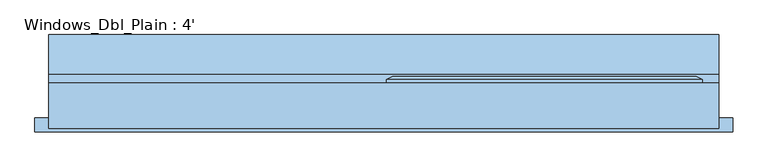
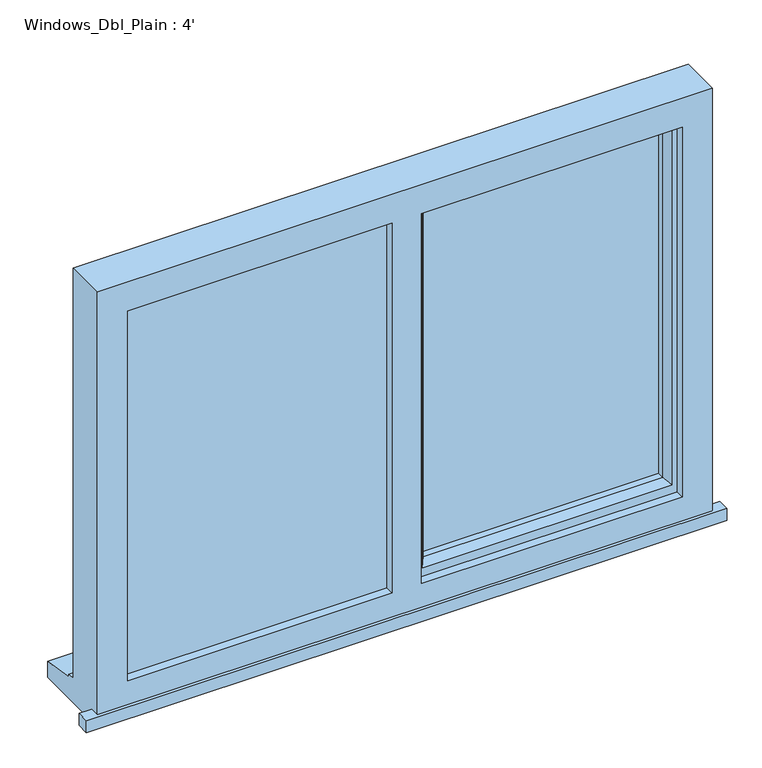
"""IFC4 building model written with IfcOpenShell, lengths in millimetres: window geometry, Windows_Dbl_Plain : 4'."""

from ifc_helpers import new_model, si_unit, frame, origin, place, context, project, spatial, polyline, outline, extrude, faceted_brep, source, transform, mapped, element, save


def windows_dbl_plain_4_4767a56f(model_context):
    return source(origin(), model_context, "Body", "SolidModel", [
        extrude(outline(polyline([(-919.6, -73.6934322), (-919.6, -48.6934322), (-894.6, -48.6934322), (-894.6, -67.3934322), (324.6, -67.3934322), (324.6, -48.6934322), (349.6, -48.6934322), (349.6, -73.6934322), (-919.6, -73.6934322)])), frame((0.0, 0.0, 1200.0), z_axis=(0.0, 0.0, 1.0), x_axis=(1.0, 0.0, 0.0)), (0.0, 0.0, 1.0), 25.0),
        faceted_brep([(-280.0, 15.6065678, 2080.0), (-280.0, 21.3800705, 2080.0), (-280.0, 21.3800705, 1253.0), (-280.0, 15.6065678, 1253.0), (-270.0, -49.3934322, 2070.0), (-270.0, 15.6065678, 2070.0), (-270.0, 15.6065678, 1263.0), (-270.0, -49.3934322, 1263.0), (-230.0, -34.9005323, 2030.0), (-240.1480377, -49.3934322, 2040.1480377), (-240.1480377, -49.3934322, 1292.8519623), (-230.0, -34.9005323, 1303.0), (-230.0, -20.3934322, 2030.0), (-230.0, -20.3934322, 1303.0), (-240.0, 3.6065678, 2040.0), (-240.0, -20.3934322, 2040.0), (-240.0, -20.3934322, 1293.0), (-240.0, 3.6065678, 1293.0), (-230.0, 21.3800705, 2030.0), (-230.0, 3.6065678, 2030.0), (-230.0, 3.6065678, 1303.0), (-230.0, 21.3800705, 1303.0), (-247.4457548, 27.1535732, 2047.4457548), (-247.4457548, 27.1535732, 1285.5542452), (-269.2153903, 27.1535732, 2069.2153903), (-269.2153903, 27.1535732, 1263.7846097), (294.6, 21.3800705, 1253.0), (294.6, 15.6065678, 1253.0), (284.6, 15.6065678, 1263.0), (284.6, -49.3934322, 1263.0), (254.7480377, -49.3934322, 1292.8519623), (244.6, -34.9005323, 1303.0), (244.6, -20.3934322, 1303.0), (254.6, -20.3934322, 1293.0), (254.6, 3.6065678, 1293.0), (244.6, 3.6065678, 1303.0), (244.6, 21.3800705, 1303.0), (262.0457548, 27.1535732, 1285.5542452), (283.8153903, 27.1535732, 1263.7846097), (294.6, 21.3800705, 2080.0), (294.6, 15.6065678, 2080.0), (284.6, 15.6065678, 2070.0), (284.6, -49.3934322, 2070.0), (254.7480377, -49.3934322, 2040.1480377), (244.6, -34.9005323, 2030.0), (244.6, -20.3934322, 2030.0), (254.6, -20.3934322, 2040.0), (254.6, 3.6065678, 2040.0), (244.6, 3.6065678, 2030.0), (244.6, 21.3800705, 2030.0), (262.0457548, 27.1535732, 2047.4457548), (283.8153903, 27.1535732, 2069.2153903)], [[[0, 1, 2, 3]], [[4, 5, 6, 7]], [[8, 9, 10, 11]], [[12, 8, 11, 13]], [[14, 15, 16, 17]], [[18, 19, 20, 21]], [[22, 18, 21, 23]], [[1, 24, 25, 2]], [[3, 2, 26, 27]], [[7, 6, 28, 29]], [[11, 10, 30, 31]], [[13, 11, 31, 32]], [[17, 16, 33, 34]], [[21, 20, 35, 36]], [[23, 21, 36, 37]], [[2, 25, 38, 26]], [[27, 26, 39, 40]], [[29, 28, 41, 42]], [[31, 30, 43, 44]], [[32, 31, 44, 45]], [[34, 33, 46, 47]], [[36, 35, 48, 49]], [[37, 36, 49, 50]], [[26, 38, 51, 39]], [[40, 39, 1, 0]], [[3, 27, 40, 0], [5, 41, 28, 6]], [[42, 41, 5, 4]], [[7, 29, 42, 4], [9, 43, 30, 10]], [[44, 43, 9, 8]], [[45, 44, 8, 12]], [[15, 46, 33, 16], [13, 32, 45, 12]], [[47, 46, 15, 14]], [[17, 34, 47, 14], [19, 48, 35, 20]], [[49, 48, 19, 18]], [[50, 49, 18, 22]], [[24, 51, 38, 25], [23, 37, 50, 22]], [[39, 51, 24, 1]]]),
        extrude(outline(polyline([(2050.0, -310.0), (2070.0, -310.0), (2070.0, -854.6), (1263.0, -854.6), (1263.0, -310.0), (1283.0, -310.0), (1283.0, -834.6), (2050.0, -834.6), (2050.0, -310.0)])), frame((0.0, -25.3934322, 0.0), z_axis=(0.0, 1.0, 0.0), x_axis=(0.0, 0.0, 1.0)), (0.0, 0.0, 1.0), 41.0),
        faceted_brep([(324.6, -67.3934322, 2110.0), (-894.6, -67.3934322, 2110.0), (-894.6, -67.3934322, 1200.0), (324.6, -67.3934322, 1200.0), (264.6, -67.3934322, 2050.0), (264.6, -67.3934322, 1275.0), (-252.0, -67.3934322, 1275.0), (-252.0, -67.3934322, 2050.0), (-310.0, -67.3934322, 2050.0), (-310.0, -67.3934322, 1275.0), (-834.6, -67.3934322, 1275.0), (-834.6, -67.3934322, 2050.0), (-894.6, 15.6065678, 2110.0), (-894.6, 15.6065678, 1251.0), (-894.6, 30.6065678, 1249.68767), (-894.6, 30.6065678, 1244.7449676), (-894.6, 103.1065678, 1233.8088847), (-894.6, 103.1065678, 1200.0), (324.6, 15.6065678, 2110.0), (324.6, 15.6065678, 1251.0), (-854.6, 15.6065678, 2070.0), (-854.6, 15.6065678, 1263.0), (-310.0, 15.6065678, 1263.0), (-310.0, 15.6065678, 2070.0), (-270.0, 15.6065678, 2070.0), (-270.0, 15.6065678, 1263.0), (284.6, 15.6065678, 1263.0), (284.6, 15.6065678, 2070.0), (-854.6, -49.3934322, 2070.0), (-854.6, -49.3934322, 1263.0), (-300.0, -49.3934322, 2070.0), (-300.0, -49.3934322, 1263.0), (-310.0, -49.3934322, 2050.0), (-834.6, -49.3934322, 2050.0), (-834.6, -49.3934322, 1275.0), (-310.0, -49.3934322, 1275.0), (-270.0, -49.3934322, 2070.0), (284.6, -49.3934322, 2070.0), (284.6, -49.3934322, 1263.0), (-270.0, -49.3934322, 1263.0), (264.6, -49.3934322, 2050.0), (-252.0, -49.3934322, 2050.0), (-252.0, -49.3934322, 1275.0), (264.6, -49.3934322, 1275.0), (-310.0, -25.3934322, 2070.0), (-300.0, -25.3934322, 2070.0), (324.6, 103.1065678, 1200.0), (324.6, 103.1065678, 1233.8088847), (324.6, 30.6065678, 1244.7449676), (324.6, 30.6065678, 1249.68767), (-300.0, -25.3934322, 1263.0), (-310.0, -25.3934322, 1263.0)], [[[0, 1, 2, 3], [4, 5, 6, 7], [8, 9, 10, 11]], [[2, 1, 12, 13, 14, 15, 16, 17]], [[13, 12, 18, 19], [20, 21, 22, 23], [24, 25, 26, 27]], [[21, 20, 28, 29]], [[28, 30, 31, 29], [32, 33, 34, 35]], [[36, 37, 38, 39], [40, 41, 42, 43]], [[33, 11, 10, 34]], [[1, 0, 18, 12]], [[28, 20, 23, 44, 45, 30]], [[27, 37, 36, 24]], [[11, 33, 32, 8]], [[40, 4, 7, 41]], [[19, 18, 0, 3, 46, 47, 48, 49]], [[27, 26, 38, 37]], [[4, 40, 43, 5]], [[45, 50, 31, 30]], [[50, 45, 44, 51]], [[51, 44, 23, 22]], [[25, 24, 36, 39]], [[41, 7, 6, 42]], [[8, 32, 35, 9]], [[46, 3, 2, 17]], [[47, 46, 17, 16]], [[48, 47, 16, 15]], [[49, 48, 15, 14]], [[19, 49, 14, 13]], [[22, 21, 29, 31, 50, 51]], [[26, 25, 39, 38]], [[6, 5, 43, 42]], [[35, 34, 10, 9]]]),
        extrude(outline(polyline([(-854.6, -25.3934322), (-300.0, -25.3934322), (-300.0, -49.3934322), (-854.6, -49.3934322), (-854.6, -25.3934322)])), frame((0.0, 0.0, 1263.0), z_axis=(0.0, 0.0, 1.0), x_axis=(1.0, 0.0, 0.0)), (0.0, 0.0, 1.0), 807.0),
        extrude(outline(polyline([(254.6, -20.3934322), (-240.0, -20.3934322), (-240.0, 3.6065678), (254.6, 3.6065678), (254.6, -20.3934322)])), frame((0.0, 0.0, 1293.0), z_axis=(0.0, 0.0, 1.0), x_axis=(1.0, 0.0, 0.0)), (0.0, 0.0, 1.0), 747.0),
    ])


if __name__ == "__main__":
    model = new_model("IFC4")
    model_context = context("Model", 3, world=origin())
    ifc_project = project(units=[si_unit("LENGTHUNIT", "METRE", prefix="MILLI")], contexts=[model_context])
    site = spatial("IfcSite", under=ifc_project)
    building = spatial("IfcBuilding", under=site)
    placement = place(None, origin())
    windows_dbl_plain_4_shape = windows_dbl_plain_4_4767a56f(model_context)
    element("IfcWindow", 1, ObjectType="Windows_Dbl_Plain : 4'", at=placement, inside=building, context=model_context, shape_type="MappedRepresentation", body=[
        mapped(windows_dbl_plain_4_shape, transform((0.0, 0.0, 0.0), x_axis=(1.0, 0.0, 0.0), y_axis=(0.0, 1.0, 0.0), z_axis=(0.0, 0.0, 1.0))),
    ])
    save(model, "model.ifc")

# Revit data of these elements
# Type "Windows_Dbl_Plain : 4'"
#   Type Mark = "56"
#   Operation = "DoublePanelVertical"
#   Construction Type Id = "GSP4R"
#   Manufacturer = "Revit"
#   Keynote = "L10"
#   Analytic Construction = "1/8 in Pilkington single glazing"
#   Wrap Layers (Ext) from Ext = 0.336286 ft
#   Wrap Layers (Int) from Ext = 0.582349 ft
#   Window Board Projection = 0.082021 ft
#   Window Board Extension = 0.082021 ft
#   Visual Light Transmittance = 0.9
#   Solar Heat Gain Coefficient = 0.78
#   Rough Width = 4.0 ft
#   Rough Height = 2.985564 ft
#   Height = 2.985564 ft
#   Width = 4.0 ft
#   Heat Transfer Coefficient (U) = 3.6886 W/(m²·K)
#   Glazing Thickness = 0.07874 ft
#   FrameOffset - External = 0.164042 ft
#   Frame Depth = 0.213255 ft
#   Default Head Height = 6.922572 ft
#   Cill Depth = 0.287073 ft
#   Cavity Closer Width = 0.164042 ft
#   Cavity Closer Offset from Ext = 0.336286 ft
#   Cavity Closer Depth = 0.278871 ft
#   Vis - Cavity Closers = yes
#   Define Thermal Properties by = 1
#   Material Trim = Window Frame
#   Material Glass = Glass
#   Material Frame = Window Frame
#   Wall Closure = (empty or 0)
# Element 1 (IfcWindow, "Windows_Dbl_Plain : 4'")
#   Materials on its faces: "Window Frame", "Glass"
# Materials
#   "Window Frame": colour RGB 249 249 249, transparency 0, Keynote = "L10", Cost = 0
#   "Glass": class "Glass", colour RGB 0 128 192, transparency 0.9, Description = "Soda Lime Glass", Cost = 0
